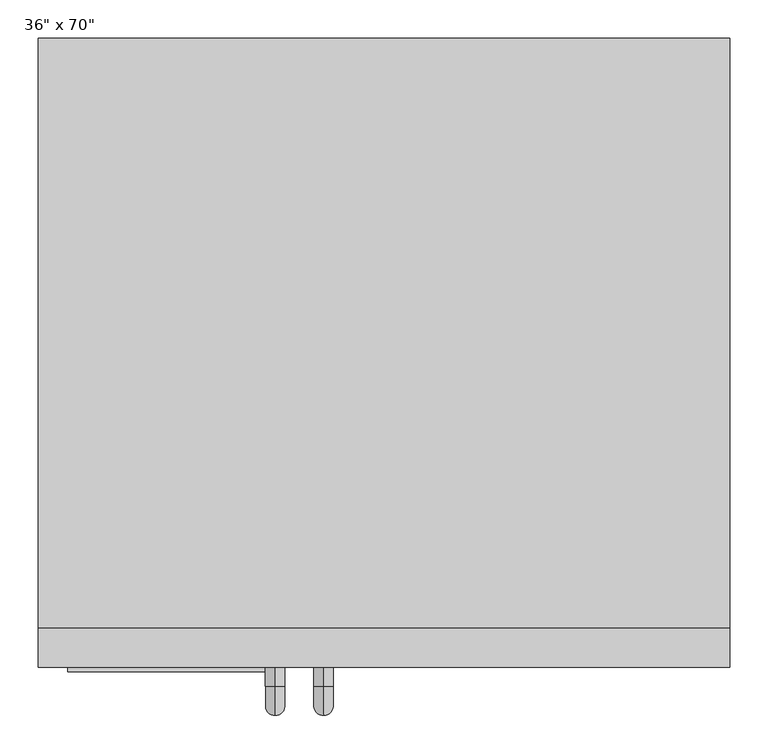
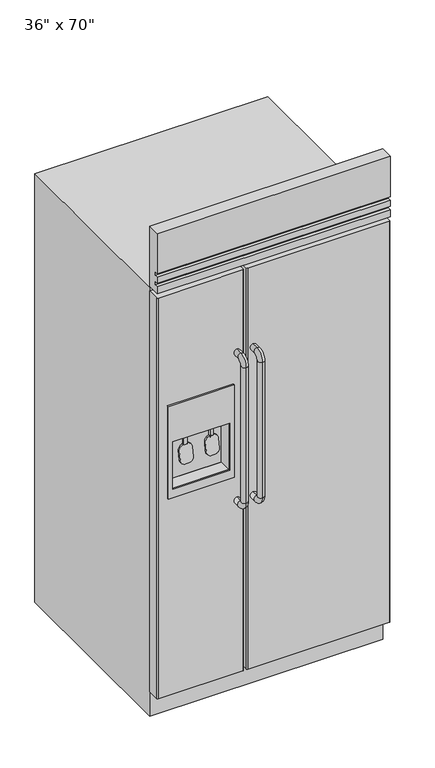
"""IFC4 building model written with IfcOpenShell, lengths in millimetres: proxy geometry."""

from ifc_helpers import new_model, si_unit, point, frame, frame_2d, origin, origin_with_axes, place, context, project, spatial, polyline, circle_curve, ellipse_curve, trimmed, segment, composite_curve, outline, extrude, faceted_brep, source, transform, mapped, element, save
from ifc_brep_helpers import plane_surface, cylinder_surface, revolved_surface, advanced_brep


def proxy_94deb4ca(model_context):
    return source(origin(), model_context, "Body", "SolidModel", [
        extrude(outline(composite_curve([segment(trimmed(circle_curve(frame_2d((31.7500242, -19.05)), 19.05), [point((31.7500242, 0.0))], [point((50.8000242, -19.05))], False, "CARTESIAN"), True, "CONTINUOUS"), segment(polyline([(50.8000242, -19.05), (50.8000242, -56.1131106)]), True, "CONTINUOUS"), segment(trimmed(circle_curve(frame_2d((31.7500242, -56.1131106)), 19.05), [point((50.8000242, -56.1131106))], [point((31.7500242, -75.1631106))], False, "CARTESIAN"), True, "CONTINUOUS"), segment(polyline([(31.7500242, -75.1631106), (19.05, -75.1631106)]), True, "CONTINUOUS"), segment(trimmed(circle_curve(frame_2d((19.05, -56.1131106)), 19.05), [point((19.05, -75.1631106))], [point((0.0, -56.1131106))], False, "CARTESIAN"), True, "CONTINUOUS"), segment(polyline([(0.0, -56.1131106), (0.0, -19.05)]), True, "CONTINUOUS"), segment(trimmed(circle_curve(frame_2d((19.05, -19.05)), 19.05), [point((0.0, -19.05))], [point((19.05, 0.0))], False, "CARTESIAN"), True, "CONTINUOUS"), segment(polyline([(19.05, 0.0), (31.7500242, 0.0)]), True, "CONTINUOUS")], self_intersect=False)), frame((-256.5190444, -433.9050771, 1103.8712429), z_axis=(0.0, -0.9890616696750606, 0.14750258838264954), x_axis=(1.0, 0.0, 0.0)), (0.0, 0.0, 1.0), 6.3500366),
        extrude(outline(polyline([(-224.7690202, -433.7760338), (-224.7690202, -440.879586), (-237.4690444, -440.879586), (-237.4690444, -433.7760338), (-224.7690202, -433.7760338)])), frame((0.0, 0.0, 1098.5109384), z_axis=(0.0, 0.0, 1.0), x_axis=(1.0, 0.0, 0.0)), (0.0, 0.0, 1.0), 44.4890616),
        extrude(outline(composite_curve([segment(trimmed(circle_curve(frame_2d((31.7500242, -19.05)), 19.05), [point((31.7500242, 0.0))], [point((50.8000242, -19.05))], False, "CARTESIAN"), True, "CONTINUOUS"), segment(polyline([(50.8000242, -19.05), (50.8000242, -56.1131106)]), True, "CONTINUOUS"), segment(trimmed(circle_curve(frame_2d((31.7500242, -56.1131106)), 19.05), [point((50.8000242, -56.1131106))], [point((31.7500242, -75.1631106))], False, "CARTESIAN"), True, "CONTINUOUS"), segment(polyline([(31.7500242, -75.1631106), (19.05, -75.1631106)]), True, "CONTINUOUS"), segment(trimmed(circle_curve(frame_2d((19.05, -56.1131106)), 19.05), [point((19.05, -75.1631106))], [point((0.0, -56.1131106))], False, "CARTESIAN"), True, "CONTINUOUS"), segment(polyline([(0.0, -56.1131106), (0.0, -19.05)]), True, "CONTINUOUS"), segment(trimmed(circle_curve(frame_2d((19.05, -19.05)), 19.05), [point((0.0, -19.05))], [point((19.05, 0.0))], False, "CARTESIAN"), True, "CONTINUOUS"), segment(polyline([(19.05, 0.0), (31.7500242, 0.0)]), True, "CONTINUOUS")], self_intersect=False)), frame((-358.1190444, -433.9050771, 1103.8712429), z_axis=(0.0, -0.9890616696750606, 0.14750258838264954), x_axis=(1.0, 0.0, 0.0)), (0.0, 0.0, 1.0), 6.3500366),
        extrude(outline(polyline([(-326.3690202, -433.7760338), (-326.3690202, -440.879586), (-339.0690444, -440.879586), (-339.0690444, -433.7760338), (-326.3690202, -433.7760338)])), frame((0.0, 0.0, 1098.5109384), z_axis=(0.0, 0.0, 1.0), x_axis=(1.0, 0.0, 0.0)), (0.0, 0.0, 1.0), 44.4890616),
        advanced_brep(
        [(-75.5440323, -452.8260346, 1435.1), (-75.5440323, -452.8260346, 1409.7), (-75.5440323, -478.2260346, 1435.1), (-75.5440323, -478.2260346, 1409.7), (-75.5440323, -490.9260346, 1397.0), (-75.5440323, -516.3260346, 1397.0), (-75.5440323, -516.3260346, 838.2), (-75.5440323, -490.9260346, 838.2), (-75.5440323, -478.2260346, 825.5), (-75.5440323, -478.2260346, 800.1), (-75.5440323, -452.8260346, 800.1), (-75.5440323, -452.8260346, 825.5)],
        [
            (0, 1, circle_curve(frame((-75.5440323, -452.8260346, 1422.4), z_axis=(0.0, 1.0, 0.0), x_axis=(0.0, 0.0, -1.0)), 12.7)),
            (1, 0, circle_curve(frame((-75.5440323, -452.8260346, 1422.4), z_axis=(0.0, 1.0, 0.0), x_axis=(0.0, 0.0, -1.0)), 12.7)),
            (0, 2),
            (2, 3, circle_curve(frame((-75.5440323, -478.2260346, 1422.4), z_axis=(0.0, 1.0, 0.0), x_axis=(0.0, 0.0, -1.0)), 12.7)),
            (3, 1),
            (3, 2, circle_curve(frame((-75.5440323, -478.2260346, 1422.4), z_axis=(0.0, 1.0, 0.0), x_axis=(0.0, 0.0, -1.0)), 12.7)),
            (4, 3, circle_curve(frame((-75.5440323, -478.2260346, 1397.0), z_axis=(-1.0, 0.0, 0.0), x_axis=(0.0, 0.0, 1.0)), 12.7)),
            (2, 5, circle_curve(frame((-75.5440323, -478.2260346, 1397.0), z_axis=(1.0, 0.0, 0.0), x_axis=(0.0, 0.0, 1.0)), 38.1)),
            (5, 4, circle_curve(frame((-75.5440323, -503.6260346, 1397.0), z_axis=(0.0, 0.0, 1.0), x_axis=(0.0, 1.0, 0.0)), 12.7)),
            (4, 5, circle_curve(frame((-75.5440323, -503.6260346, 1397.0), z_axis=(0.0, 0.0, 1.0), x_axis=(0.0, 1.0, 0.0)), 12.7)),
            (5, 6),
            (6, 7, circle_curve(frame((-75.5440323, -503.6260346, 838.2), z_axis=(0.0, 0.0, 1.0), x_axis=(0.0, 1.0, 0.0)), 12.7)),
            (7, 4),
            (7, 6, circle_curve(frame((-75.5440323, -503.6260346, 838.2), z_axis=(0.0, 0.0, 1.0), x_axis=(0.0, 1.0, 0.0)), 12.7)),
            (8, 7, circle_curve(frame((-75.5440323, -478.2260346, 838.2), z_axis=(-1.0, 0.0, 0.0), x_axis=(0.0, -1.0, 0.0)), 12.7)),
            (6, 9, circle_curve(frame((-75.5440323, -478.2260346, 838.2), z_axis=(1.0, 0.0, 0.0), x_axis=(0.0, -1.0, 0.0)), 38.1)),
            (9, 8, circle_curve(frame((-75.5440323, -478.2260346, 812.8), z_axis=(0.0, -1.0, 0.0), x_axis=(0.0, 0.0, 1.0)), 12.7)),
            (8, 9, circle_curve(frame((-75.5440323, -478.2260346, 812.8), z_axis=(0.0, -1.0, 0.0), x_axis=(0.0, 0.0, 1.0)), 12.7)),
            (10, 11, circle_curve(frame((-75.5440323, -452.8260346, 812.8), z_axis=(0.0, 1.0, 0.0), x_axis=(0.0, 0.0, 1.0)), 12.7)),
            (11, 10, circle_curve(frame((-75.5440323, -452.8260346, 812.8), z_axis=(0.0, 1.0, 0.0), x_axis=(0.0, 0.0, 1.0)), 12.7)),
            (9, 10),
            (11, 8),
        ],
        [
            plane_surface(frame((-75.5440323, -452.8260346, 1422.4), z_axis=(0.0, 1.0, 0.0), x_axis=(1.0, 0.0, 0.0))),
            cylinder_surface(frame((-75.5440323, -452.8260346, 1422.4), z_axis=(0.0, 1.0, 0.0), x_axis=(0.0, 0.0, -1.0)), 12.7),
            revolved_surface(trimmed(ellipse_curve(frame((-75.5440323, -478.2260346, 1422.4), z_axis=(0.0, 1.0, 0.0), x_axis=(0.0, 0.0, -1.0)), 12.7, 12.7), [point((-75.5440323, -478.2260346, 1435.1))], [point((-75.5440323, -478.2260346, 1409.7))], True, "CARTESIAN"), (-75.5440323, -478.2260346, 1397.0), (1.0, 0.0, 0.0)),
            revolved_surface(trimmed(ellipse_curve(frame((-75.5440323, -478.2260346, 1422.4), z_axis=(0.0, 1.0, 0.0), x_axis=(0.0, 0.0, -1.0)), 12.7, 12.7), [point((-75.5440323, -478.2260346, 1409.7))], [point((-75.5440323, -478.2260346, 1435.1))], True, "CARTESIAN"), (-75.5440323, -478.2260346, 1397.0), (1.0, 0.0, 0.0)),
            cylinder_surface(frame((-75.5440323, -503.6260346, 1397.0), z_axis=(0.0, 0.0, 1.0), x_axis=(0.0, 1.0, 0.0)), 12.7),
            revolved_surface(trimmed(ellipse_curve(frame((-75.5440323, -503.6260346, 838.2), z_axis=(0.0, 0.0, 1.0), x_axis=(0.0, 1.0, 0.0)), 12.7, 12.7), [point((-75.5440323, -516.3260346, 838.2))], [point((-75.5440323, -490.9260346, 838.2))], True, "CARTESIAN"), (-75.5440323, -478.2260346, 838.2), (1.0, 0.0, 0.0)),
            revolved_surface(trimmed(ellipse_curve(frame((-75.5440323, -503.6260346, 838.2), z_axis=(0.0, 0.0, 1.0), x_axis=(0.0, 1.0, 0.0)), 12.7, 12.7), [point((-75.5440323, -490.9260346, 838.2))], [point((-75.5440323, -516.3260346, 838.2))], True, "CARTESIAN"), (-75.5440323, -478.2260346, 838.2), (1.0, 0.0, 0.0)),
            plane_surface(frame((-75.5440323, -452.8260346, 812.8), z_axis=(0.0, 1.0, 0.0), x_axis=(1.0, 0.0, 0.0))),
            cylinder_surface(frame((-75.5440323, -478.2260346, 812.8), z_axis=(0.0, -1.0, 0.0), x_axis=(0.0, 0.0, 1.0)), 12.7),
        ],
        [
            (0, [[1, 2]]),
            (1, [[-1, 3, 4, 5]]),
            (1, [[-2, -5, 6, -3]]),
            (2, [[7, -4, 8, 9]]),
            (3, [[-8, -6, -7, 10]]),
            (4, [[-9, 11, 12, 13]]),
            (4, [[-10, -13, 14, -11]]),
            (5, [[15, -12, 16, 17]]),
            (6, [[-16, -14, -15, 18]]),
            (7, [[19, 20]]),
            (8, [[-17, 21, -20, 22]]),
            (8, [[-18, -22, -19, -21]]),
        ],
    ),
        advanced_brep(
        [(-139.0440323, -452.8260346, 1435.1), (-139.0440323, -452.8260346, 1409.7), (-139.0440323, -478.2260346, 1435.1), (-139.0440323, -478.2260346, 1409.7), (-139.0440323, -490.9260346, 1397.0), (-139.0440323, -516.3260346, 1397.0), (-139.0440323, -516.3260346, 838.2), (-139.0440323, -490.9260346, 838.2), (-139.0440323, -478.2260346, 825.5), (-139.0440323, -478.2260346, 800.1), (-139.0440323, -452.8260346, 800.1), (-139.0440323, -452.8260346, 825.5)],
        [
            (0, 1, circle_curve(frame((-139.0440323, -452.8260346, 1422.4), z_axis=(0.0, 1.0, 0.0), x_axis=(0.0, 0.0, -1.0)), 12.7)),
            (1, 0, circle_curve(frame((-139.0440323, -452.8260346, 1422.4), z_axis=(0.0, 1.0, 0.0), x_axis=(0.0, 0.0, -1.0)), 12.7)),
            (0, 2),
            (2, 3, circle_curve(frame((-139.0440323, -478.2260346, 1422.4), z_axis=(0.0, 1.0, 0.0), x_axis=(0.0, 0.0, -1.0)), 12.7)),
            (3, 1),
            (3, 2, circle_curve(frame((-139.0440323, -478.2260346, 1422.4), z_axis=(0.0, 1.0, 0.0), x_axis=(0.0, 0.0, -1.0)), 12.7)),
            (4, 3, circle_curve(frame((-139.0440323, -478.2260346, 1397.0), z_axis=(-1.0, 0.0, 0.0), x_axis=(0.0, 0.0, 1.0)), 12.7)),
            (2, 5, circle_curve(frame((-139.0440323, -478.2260346, 1397.0), z_axis=(1.0, 0.0, 0.0), x_axis=(0.0, 0.0, 1.0)), 38.1)),
            (5, 4, circle_curve(frame((-139.0440323, -503.6260346, 1397.0), z_axis=(0.0, 0.0, 1.0), x_axis=(0.0, 1.0, 0.0)), 12.7)),
            (4, 5, circle_curve(frame((-139.0440323, -503.6260346, 1397.0), z_axis=(0.0, 0.0, 1.0), x_axis=(0.0, 1.0, 0.0)), 12.7)),
            (5, 6),
            (6, 7, circle_curve(frame((-139.0440323, -503.6260346, 838.2), z_axis=(0.0, 0.0, 1.0), x_axis=(0.0, 1.0, 0.0)), 12.7)),
            (7, 4),
            (7, 6, circle_curve(frame((-139.0440323, -503.6260346, 838.2), z_axis=(0.0, 0.0, 1.0), x_axis=(0.0, 1.0, 0.0)), 12.7)),
            (8, 7, circle_curve(frame((-139.0440323, -478.2260346, 838.2), z_axis=(-1.0, 0.0, 0.0), x_axis=(0.0, -1.0, 0.0)), 12.7)),
            (6, 9, circle_curve(frame((-139.0440323, -478.2260346, 838.2), z_axis=(1.0, 0.0, 0.0), x_axis=(0.0, -1.0, 0.0)), 38.1)),
            (9, 8, circle_curve(frame((-139.0440323, -478.2260346, 812.8), z_axis=(0.0, -1.0, 0.0), x_axis=(0.0, 0.0, 1.0)), 12.7)),
            (8, 9, circle_curve(frame((-139.0440323, -478.2260346, 812.8), z_axis=(0.0, -1.0, 0.0), x_axis=(0.0, 0.0, 1.0)), 12.7)),
            (10, 11, circle_curve(frame((-139.0440323, -452.8260346, 812.8), z_axis=(0.0, 1.0, 0.0), x_axis=(0.0, 0.0, 1.0)), 12.7)),
            (11, 10, circle_curve(frame((-139.0440323, -452.8260346, 812.8), z_axis=(0.0, 1.0, 0.0), x_axis=(0.0, 0.0, 1.0)), 12.7)),
            (9, 10),
            (11, 8),
        ],
        [
            plane_surface(frame((-139.0440323, -452.8260346, 1422.4), z_axis=(0.0, 1.0, 0.0), x_axis=(1.0, 0.0, 0.0))),
            cylinder_surface(frame((-139.0440323, -452.8260346, 1422.4), z_axis=(0.0, 1.0, 0.0), x_axis=(0.0, 0.0, -1.0)), 12.7),
            revolved_surface(trimmed(ellipse_curve(frame((-139.0440323, -478.2260346, 1422.4), z_axis=(0.0, 1.0, 0.0), x_axis=(0.0, 0.0, -1.0)), 12.7, 12.7), [point((-139.0440323, -478.2260346, 1435.1))], [point((-139.0440323, -478.2260346, 1409.7))], True, "CARTESIAN"), (-139.0440323, -478.2260346, 1397.0), (1.0, 0.0, 0.0)),
            revolved_surface(trimmed(ellipse_curve(frame((-139.0440323, -478.2260346, 1422.4), z_axis=(0.0, 1.0, 0.0), x_axis=(0.0, 0.0, -1.0)), 12.7, 12.7), [point((-139.0440323, -478.2260346, 1409.7))], [point((-139.0440323, -478.2260346, 1435.1))], True, "CARTESIAN"), (-139.0440323, -478.2260346, 1397.0), (1.0, 0.0, 0.0)),
            cylinder_surface(frame((-139.0440323, -503.6260346, 1397.0), z_axis=(0.0, 0.0, 1.0), x_axis=(0.0, 1.0, 0.0)), 12.7),
            revolved_surface(trimmed(ellipse_curve(frame((-139.0440323, -503.6260346, 838.2), z_axis=(0.0, 0.0, 1.0), x_axis=(0.0, 1.0, 0.0)), 12.7, 12.7), [point((-139.0440323, -516.3260346, 838.2))], [point((-139.0440323, -490.9260346, 838.2))], True, "CARTESIAN"), (-139.0440323, -478.2260346, 838.2), (1.0, 0.0, 0.0)),
            revolved_surface(trimmed(ellipse_curve(frame((-139.0440323, -503.6260346, 838.2), z_axis=(0.0, 0.0, 1.0), x_axis=(0.0, 1.0, 0.0)), 12.7, 12.7), [point((-139.0440323, -490.9260346, 838.2))], [point((-139.0440323, -516.3260346, 838.2))], True, "CARTESIAN"), (-139.0440323, -478.2260346, 838.2), (1.0, 0.0, 0.0)),
            plane_surface(frame((-139.0440323, -452.8260346, 812.8), z_axis=(0.0, 1.0, 0.0), x_axis=(1.0, 0.0, 0.0))),
            cylinder_surface(frame((-139.0440323, -478.2260346, 812.8), z_axis=(0.0, -1.0, 0.0), x_axis=(0.0, 0.0, 1.0)), 12.7),
        ],
        [
            (0, [[1, 2]]),
            (1, [[-1, 3, 4, 5]]),
            (1, [[-2, -5, 6, -3]]),
            (2, [[7, -4, 8, 9]]),
            (3, [[-8, -6, -7, 10]]),
            (4, [[-9, 11, 12, 13]]),
            (4, [[-10, -13, 14, -11]]),
            (5, [[15, -12, 16, 17]]),
            (6, [[-16, -14, -15, 18]]),
            (7, [[19, 20]]),
            (8, [[-17, 21, -20, 22]]),
            (8, [[-18, -22, -19, -21]]),
        ],
    ),
        extrude(outline(polyline([(-402.0260346, 2019.3), (-402.0260346, 1771.7107521), (-452.8260346, 1771.7107521), (-452.8260346, 1800.0321339), (-440.1260346, 1800.0321339), (-440.1260346, 1814.1927521), (-452.8260346, 1814.1927521), (-452.8260346, 1838.9740883), (-440.1260346, 1838.9740883), (-440.1260346, 1853.1347065), (-452.8260346, 1853.1347065), (-452.8260346, 2019.3), (-402.0260346, 2019.3)])), frame((-450.1940323, 0.0, 0.0), z_axis=(1.0, 0.0, 0.0), x_axis=(0.0, 1.0, 0.0)), (0.0, 0.0, 1.0), 908.05),
        advanced_brep(
        [(-113.6440323, -402.0260346, 1752.6), (-450.1940323, -402.0260346, 1752.6), (-450.1940323, -449.6510346, 1752.6), (-447.0190323, -452.8260346, 1752.6), (-116.8190323, -452.8260346, 1752.6), (-113.6440323, -449.6510346, 1752.6), (-113.6440323, -402.0260346, 101.6), (-113.6440323, -449.6510346, 101.6), (-116.8190323, -452.8260346, 101.6), (-447.0190323, -452.8260346, 101.6), (-450.1940323, -449.6510346, 101.6), (-450.1940323, -402.0260346, 101.6), (-171.3540998, -402.0260346, 1144.5112749), (-392.4839647, -402.0260346, 1144.5112749), (-392.4839647, -402.0260346, 949.8017208), (-171.3540998, -402.0260346, 949.8017208), (-392.4839647, -452.8260346, 1144.5112749), (-171.3540998, -452.8260346, 1144.5112749), (-171.3540998, -452.8260346, 949.8017208), (-392.4839647, -452.8260346, 949.8017208)],
        [
            (0, 1),
            (1, 2),
            (2, 3, circle_curve(frame((-447.0190323, -449.6510346, 1752.6), z_axis=(0.0, 0.0, 1.0), x_axis=(0.0, -1.0, 0.0)), 3.175)),
            (3, 4),
            (4, 5, circle_curve(frame((-116.8190323, -449.6510346, 1752.6), z_axis=(0.0, 0.0, 1.0), x_axis=(0.0, -1.0, 0.0)), 3.175)),
            (5, 0),
            (6, 7),
            (7, 8, circle_curve(frame((-116.8190323, -449.6510346, 101.6), z_axis=(0.0, 0.0, -1.0), x_axis=(0.0, -1.0, 0.0)), 3.175)),
            (8, 9),
            (9, 10, circle_curve(frame((-447.0190323, -449.6510346, 101.6), z_axis=(0.0, 0.0, -1.0), x_axis=(0.0, -1.0, 0.0)), 3.175)),
            (10, 11),
            (11, 6),
            (0, 6),
            (11, 1),
            (12, 13),
            (13, 14),
            (14, 15),
            (15, 12),
            (10, 2),
            (9, 3),
            (8, 4),
            (16, 17),
            (17, 18),
            (18, 19),
            (19, 16),
            (7, 5),
            (12, 17),
            (16, 13),
            (19, 14),
            (18, 15),
        ],
        [
            plane_surface(frame((-450.1940323, -402.0260346, 1752.6), z_axis=(0.0, 0.0, 1.0), x_axis=(-1.0, 0.0, 0.0))),
            plane_surface(frame((-450.1940323, -402.0260346, 101.6), z_axis=(0.0, 0.0, -1.0), x_axis=(1.0, 0.0, 0.0))),
            plane_surface(frame((-113.6440323, -402.0260346, 1752.6), z_axis=(0.0, 1.0, 0.0), x_axis=(0.0, 0.0, -1.0))),
            plane_surface(frame((-450.1940323, -402.0260346, 1752.6), z_axis=(-1.0, 0.0, 0.0), x_axis=(0.0, 0.0, -1.0))),
            cylinder_surface(frame((-447.0190323, -449.6510346, 101.6), z_axis=(0.0, 0.0, 1.0), x_axis=(0.0, -1.0, 0.0)), 3.175),
            plane_surface(frame((-447.0190323, -452.8260346, 1752.6), z_axis=(0.0, -1.0, 0.0), x_axis=(0.0, 0.0, -1.0))),
            cylinder_surface(frame((-116.8190323, -449.6510346, 101.6), z_axis=(0.0, 0.0, 1.0), x_axis=(0.0, -1.0, 0.0)), 3.175),
            plane_surface(frame((-113.6440323, -449.6510346, 1752.6), z_axis=(1.0, 0.0, 0.0), x_axis=(0.0, 0.0, -1.0))),
            plane_surface(frame((-171.3540998, -459.1760346, 1144.5112749), z_axis=(0.0, 0.0, -1.0), x_axis=(0.0, 1.0, 0.0))),
            plane_surface(frame((-392.4839647, -459.1760346, 1144.5112749), z_axis=(1.0, 0.0, 0.0), x_axis=(0.0, 1.0, 0.0))),
            plane_surface(frame((-392.4839647, -459.1760346, 949.8017208), z_axis=(0.0, 0.0, 1.0), x_axis=(0.0, 1.0, 0.0))),
            plane_surface(frame((-171.3540998, -459.1760346, 949.8017208), z_axis=(-1.0, 0.0, 0.0), x_axis=(0.0, 1.0, 0.0))),
        ],
        [
            (0, [[1, 2, 3, 4, 5, 6]]),
            (1, [[7, 8, 9, 10, 11, 12]]),
            (2, [[-1, 13, -12, 14], [15, 16, 17, 18]]),
            (3, [[-2, -14, -11, 19]]),
            (4, [[-3, -19, -10, 20]]),
            (5, [[-4, -20, -9, 21], [22, 23, 24, 25]]),
            (6, [[-5, -21, -8, 26]]),
            (7, [[-6, -26, -7, -13]]),
            (8, [[27, -22, 28, -15]]),
            (9, [[-28, -25, 29, -16]]),
            (10, [[-29, -24, 30, -17]]),
            (11, [[-27, -18, -30, -23]]),
        ],
    ),
        faceted_brep([(-152.7858292, -285.0030875, 1296.7387564), (-152.7858292, -285.0030875, 914.4), (-411.0522354, -285.0030875, 914.4), (-411.0522354, -285.0030875, 1296.7387564), (-152.7858292, -459.1760346, 1296.7387564), (-411.0522354, -459.1760346, 1296.7387564), (-411.0522354, -459.1760346, 914.4), (-152.7858292, -459.1760346, 914.4), (-392.4839647, -459.1760346, 1144.5112749), (-171.3540998, -459.1760346, 1144.5112749), (-171.3540998, -459.1760346, 949.8017208), (-392.4839647, -459.1760346, 949.8017208), (-171.3540998, -383.3655665, 1144.5112749), (-392.4839647, -383.3655665, 1144.5112749), (-392.4839647, -383.3655665, 949.8017208), (-171.3540998, -383.3655665, 949.8017208)], [[[0, 1, 2, 3]], [[4, 5, 6, 7], [8, 9, 10, 11]], [[1, 0, 4, 7]], [[2, 1, 7, 6]], [[3, 2, 6, 5]], [[0, 3, 5, 4]], [[12, 13, 14, 15]], [[13, 12, 9, 8]], [[14, 13, 8, 11]], [[15, 14, 11, 10]], [[12, 15, 10, 9]]]),
        extrude(outline(composite_curve([segment(polyline([(457.8559677, -402.0260346), (457.8559677, -449.6510346)]), True, "CONTINUOUS"), segment(trimmed(circle_curve(frame_2d((454.6809677, -449.6510346)), 3.175), [point((457.8559677, -449.6510346))], [point((454.6809677, -452.8260346))], False, "CARTESIAN"), True, "CONTINUOUS"), segment(polyline([(454.6809677, -452.8260346), (-97.7690323, -452.8260346)]), True, "CONTINUOUS"), segment(trimmed(circle_curve(frame_2d((-97.7690323, -449.6510346)), 3.175), [point((-97.7690323, -452.8260346))], [point((-100.9440323, -449.6510346))], False, "CARTESIAN"), True, "CONTINUOUS"), segment(polyline([(-100.9440323, -449.6510346), (-100.9440323, -402.0260346), (457.8559677, -402.0260346)]), True, "CONTINUOUS")], self_intersect=False)), frame((0.0, 0.0, 101.6), z_axis=(0.0, 0.0, 1.0), x_axis=(1.0, 0.0, 0.0)), (0.0, 0.0, 1.0), 1651.0),
        extrude(outline(polyline([(457.8559677, 372.6739654), (457.8559677, -402.0260346), (-450.1940323, -402.0260346), (-450.1940323, 372.6739654), (457.8559677, 372.6739654)])), origin_with_axes(), (0.0, 0.0, 1.0), 1765.3),
    ])


if __name__ == "__main__":
    model = new_model("IFC4")
    model_context = context("Model", 3, world=origin())
    ifc_project = project(units=[si_unit("LENGTHUNIT", "METRE", prefix="MILLI")], contexts=[model_context])
    site = spatial("IfcSite", under=ifc_project)
    building = spatial("IfcBuilding", under=site)
    placement = place(None, origin())
    proxy_shape = proxy_94deb4ca(model_context)
    element("IfcBuildingElementProxy", 1, Name="36\" x 70\"", ObjectType="36\" x 70\"", at=placement, inside=building, context=model_context, shape_type="MappedRepresentation", body=[
        mapped(proxy_shape, transform((0.0, 0.0, 0.0), x_axis=(1.0, 0.0, 0.0), y_axis=(0.0, 1.0, 0.0), z_axis=(0.0, 0.0, 1.0))),
    ])
    save(model, "model.ifc")

# Revit data of these elements
# Type "36\" x 70\""
#   URL = "\r\n"
#   Label = "REF."
#   Unit_Width = 2' - 11 3/4"
#   Unit_Height = 5' - 9 1/2"
#   Unit_Depth = 2' - 8 1/2"
#   Cover_Height = 0' - 10"
#   Rigth_Door_width = 1' - 10"
#   Door_Height = 5' - 5"
#   Bottom_of_dispenser = 3' - 0"
#   Base_Height = 0' - 3 1/2"
#   Material = Metal - Stainless Steel
#   Default Elevation = 0
#   Model = ""
#   Manufacturer = ""
#   Description = (empty or 0)
#   Assembly Code = ""
# Element 1 (IfcBuildingElementProxy, "36\" x 70\"")
#   Materials on its faces: "Metal - Stainless Steel", "High Gloss Black"
# Materials
#   "Metal - Stainless Steel": colour RGB 189 187 185, transparency 0
#   "High Gloss Black": class "Metal", colour RGB 70 70 70, transparency 0
